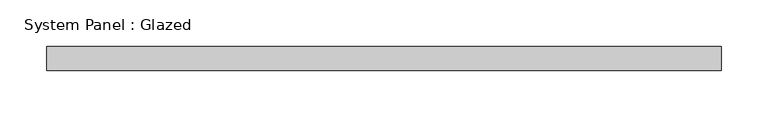
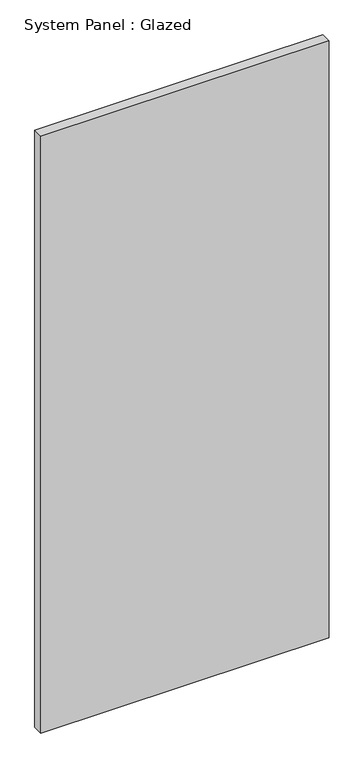
"""IFC4 building model written with IfcOpenShell, lengths in millimetres: plate geometry, System Panel : Glazed."""

from ifc_helpers import new_model, si_unit, origin, origin_with_axes, place, context, project, spatial, polyline, outline, extrude, source, transform, mapped, element, save


def system_panel_glazed_30ed1ba4(model_context):
    return source(origin(), model_context, "Body", "SweptSolid", [
        extrude(outline(polyline([(358.775, 19.05), (-358.775, 19.05), (-358.775, 44.45), (358.775, 44.45), (358.775, 19.05)])), origin_with_axes(), (0.0, 0.0, 1.0), 1570.4525236),
    ])


if __name__ == "__main__":
    model = new_model("IFC4")
    model_context = context("Model", 3, world=origin())
    ifc_project = project(units=[si_unit("LENGTHUNIT", "METRE", prefix="MILLI")], contexts=[model_context])
    site = spatial("IfcSite", under=ifc_project)
    building = spatial("IfcBuilding", under=site)
    placement = place(None, origin())
    system_panel_glazed_shape = system_panel_glazed_30ed1ba4(model_context)
    element("IfcPlate", 1, ObjectType="System Panel : Glazed", at=placement, inside=building, context=model_context, shape_type="MappedRepresentation", body=[
        mapped(system_panel_glazed_shape, transform((0.0, 0.0, 0.0), x_axis=(1.0, 0.0, 0.0), y_axis=(0.0, 1.0, 0.0), z_axis=(0.0, 0.0, 1.0))),
    ])
    save(model, "model.ifc")

# Revit data of these elements
# Type "System Panel : Glazed"
#   Construction Type Id = "GSP4R"
#   Analytic Construction = "1/8 in Pilkington single glazing"
#   Visual Light Transmittance = 0.9
#   Solar Heat Gain Coefficient = 0.86
#   Heat Transfer Coefficient (U) = 1.18115 BTU/(h·ft²·°F)
#   Define Thermal Properties by = 1
# Element 1 (IfcPlate, "System Panel : Glazed")
#   Materials on its faces: "Glass"
# Materials
#   "Glass": class "Glass", colour RGB 0 128 192, transparency 0.75, Description = "Soda Lime Glass", Cost = 0
